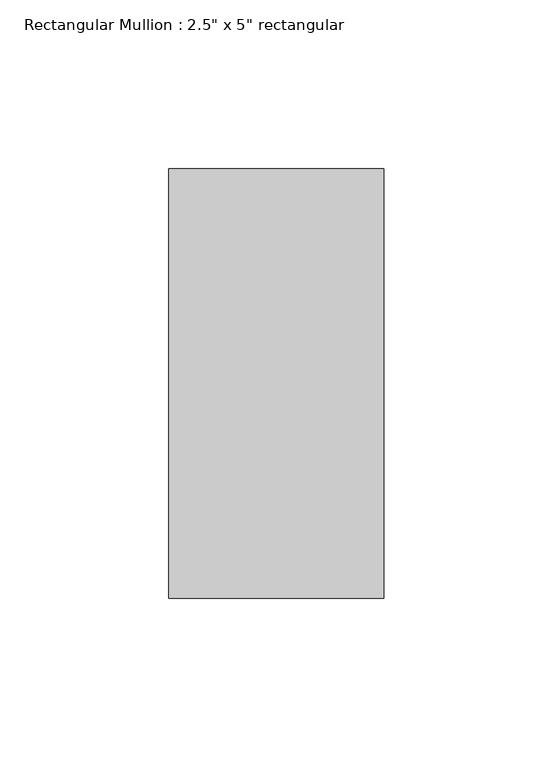
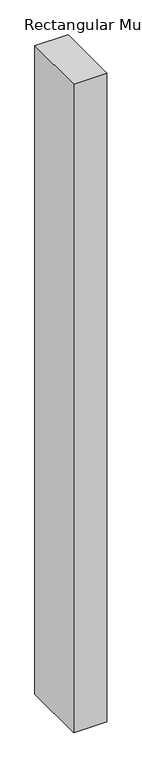
"""IFC4 building model written with IfcOpenShell, lengths in millimetres: member geometry."""

from ifc_helpers import new_model, si_unit, frame, origin, place, context, project, spatial, polyline, outline, extrude, source, transform, mapped, element, save


def member_37fe5cbd(model_context):
    return source(origin(), model_context, "Body", "SweptSolid", [
        extrude(outline(polyline([(31.75, 63.5), (31.75, -63.5), (-31.75, -63.5), (-31.75, 63.5), (31.75, 63.5)])), frame((0.0, 0.0, -1301.7500001), z_axis=(0.0, 0.0, 1.0), x_axis=(1.0, 0.0, 0.0)), (0.0, 0.0, 1.0), 1301.7500001),
    ])


if __name__ == "__main__":
    model = new_model("IFC4")
    model_context = context("Model", 3, world=origin())
    ifc_project = project(units=[si_unit("LENGTHUNIT", "METRE", prefix="MILLI")], contexts=[model_context])
    site = spatial("IfcSite", under=ifc_project)
    building = spatial("IfcBuilding", under=site)
    placement = place(None, origin())
    member_shape = member_37fe5cbd(model_context)
    element("IfcMember", 1, ObjectType="Rectangular Mullion : 2.5\" x 5\" rectangular", at=placement, inside=building, context=model_context, shape_type="MappedRepresentation", body=[
        mapped(member_shape, transform((0.0, 0.0, 0.0), x_axis=(1.0, 0.0, 0.0), y_axis=(0.0, 1.0, 0.0), z_axis=(0.0, 0.0, 1.0))),
    ])
    save(model, "model.ifc")

# Revit data of these elements
# Type "Rectangular Mullion : 2.5\" x 5\" rectangular"
#   built-in parameter 1007304 = 0.416667 (stored number, unit not read)
#   built-in parameter 1007301 = 0.104167 (stored number, unit not read)
#   built-in parameter 1007300 = 0.104167 (stored number, unit not read)
# Element 1 (IfcMember, "Rectangular Mullion : 2.5\" x 5\" rectangular")
#   Materials on its faces: "Aluminum"
# Materials
#   "Aluminum": class "Metal", colour RGB 247 247 247, transparency 0, Description = "Aluminum 6061", Cost = 0
